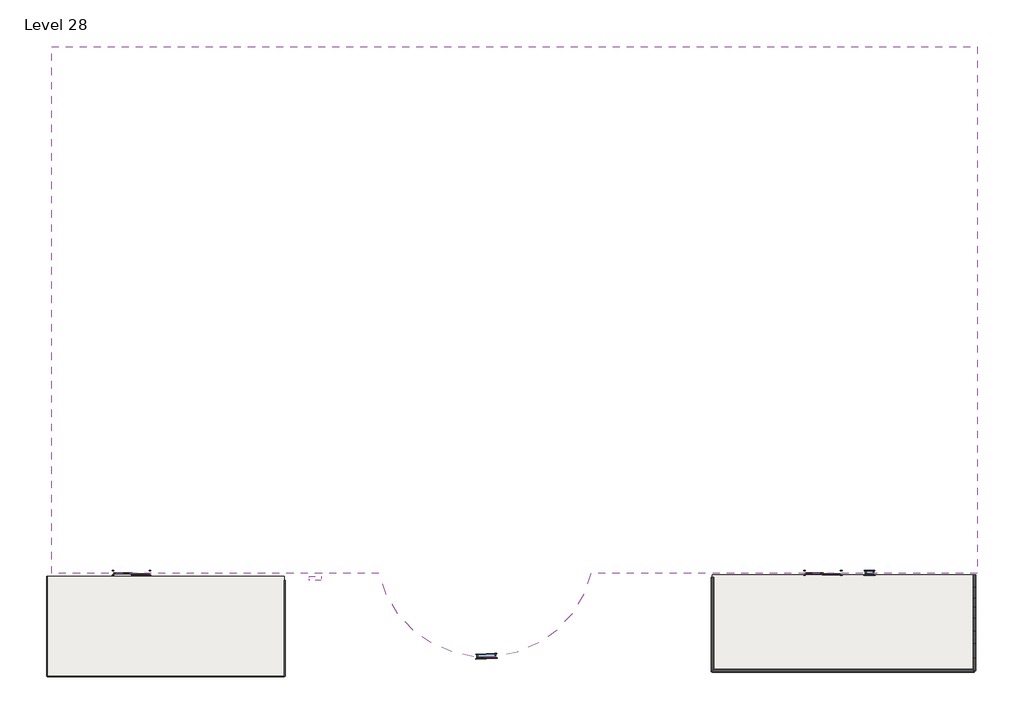
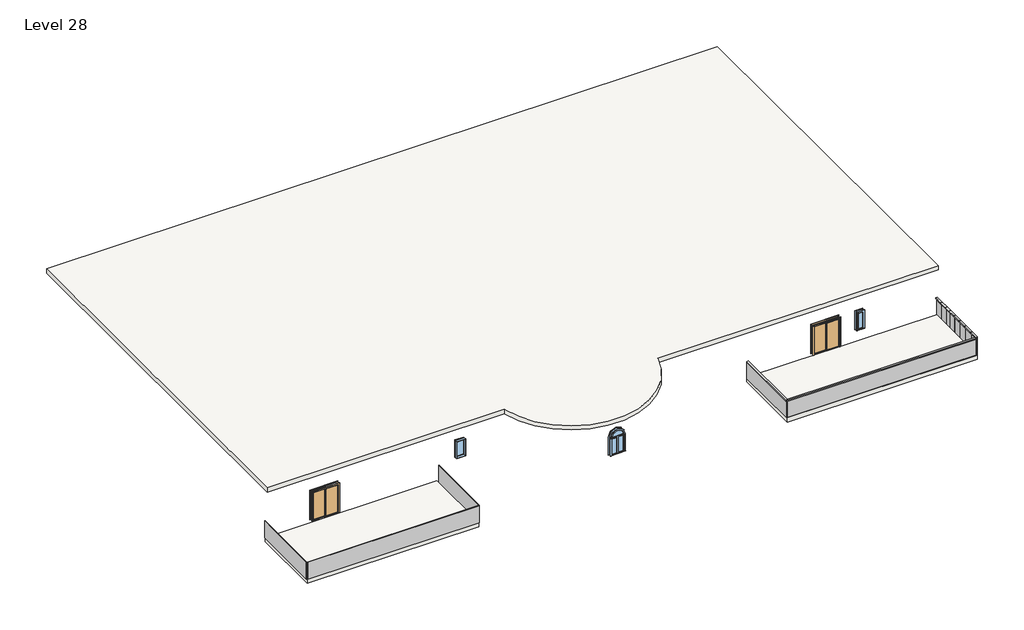
# One storey: 13 plates, 11 members, 3 slabs, 3 windows, 2 doors.
"""IFC4 building model written with IfcOpenShell, lengths in millimetres."""

from ifc_helpers import new_model, si_unit, point, frame, frame_2d, origin, place, context, project, spatial, polyline, circle_curve, trimmed, segment, composite_curve, outline, extrude, transform, mapped, element, save
from components import door_076b30e0, member_75074519, member_47bfaf8a, member_baaa0d74, member_cd3c8de8, member_7cfea1b5, member_50cacee6, member_5e365d0c, member_ae70dd35, member_19d8ec5e, system_panel_glazed_febc6b86, system_panel_glazed_7af1c9c3, system_panel_glazed_05863204, system_panel_glazed_4d5e8b0b, system_panel_glazed_a854efd3, system_panel_glazed_6a65e850, system_panel_glazed_b34e3459, system_panel_glazed_f1530dac, system_panel_glazed_53c2349a, system_panel_glazed_0853085d, system_panel_glazed_62bdce80, window_cf4adaea, window_a765b88f, window_80bd9af0

model = new_model("IFC4")

# Units and contexts
model_context = context("Model", 3, world=origin())
ifc_project = project(units=[si_unit("LENGTHUNIT", "METRE", prefix="MILLI")], contexts=[model_context])

# Site, building, storey
site = spatial("IfcSite", under=ifc_project)
building = spatial("IfcBuilding", under=site)
storey = spatial("IfcBuildingStorey", under=building, Name="Level 28", Elevation=46634.4)

# Doors
placement = place(None, origin())
door_shape = door_076b30e0(model_context)
element("IfcDoor", 1, ObjectType="Door-Double-Sliding : 68\" x 80\"", at=placement, inside=storey, context=model_context, shape_type="MappedRepresentation", body=[
    mapped(door_shape, transform((-15759.785279, -12227.7237084, 46634.4), x_axis=(-1.0, 0.0, 0.0), y_axis=(0.0, -1.0, 0.0), z_axis=(0.0, 0.0, 1.0))),
])
element("IfcDoor", 2, ObjectType="Door-Double-Sliding : 68\" x 80\"", at=placement, inside=storey, context=model_context, shape_type="MappedRepresentation", body=[
    mapped(door_shape, transform((18073.014721, -12227.7237084, 46634.4), x_axis=(-1.0, 0.0, 0.0), y_axis=(0.0, -1.0, 0.0), z_axis=(0.0, 0.0, 1.0))),
])

# Members
member_shape = member_75074519(model_context)
element("IfcMember", 3, ObjectType="Rectangular Mullion : 2.5\" x 5\" rectangular", at=placement, inside=storey, context=model_context, shape_type="MappedRepresentation", body=[
    mapped(member_shape, transform((25489.814721, -17135.5727399, 47853.6), x_axis=(1.0, 0.0, 0.0), y_axis=(0.0, 1.0, 0.0), z_axis=(0.0, 0.0, 1.0))),
])
member_2_shape = member_47bfaf8a(model_context)
element("IfcMember", 4, ObjectType="Rectangular Mullion : 2.5\" x 5\" rectangular", at=placement, inside=storey, context=model_context, shape_type="MappedRepresentation", body=[
    mapped(member_2_shape, transform((25489.814721, -15179.7727399, 47853.6), x_axis=(0.0, 0.0, 1.0), y_axis=(-1.0, 0.0, 0.0), z_axis=(0.0, -1.0, 0.0))),
])
member_3_shape = member_baaa0d74(model_context)
element("IfcMember", 5, ObjectType="Rectangular Mullion : 2.5\" x 5\" rectangular", at=placement, inside=storey, context=model_context, shape_type="MappedRepresentation", body=[
    mapped(member_3_shape, transform((12667.5594464, -12557.9237084, 47853.6), x_axis=(0.0, 0.0, 1.0), y_axis=(1.0, 0.0, 0.0), z_axis=(0.0, 1.0, 0.0))),
])
member_4_shape = member_cd3c8de8(model_context)
element("IfcMember", 6, ObjectType="Rectangular Mullion : 2.5\" x 5\" rectangular", at=placement, inside=storey, context=model_context, shape_type="MappedRepresentation", body=[
    mapped(member_4_shape, transform((25489.814721, -13030.6482241, 47853.6), x_axis=(0.0, 0.0, 1.0), y_axis=(-1.0, 0.0, 0.0), z_axis=(0.0, -1.0, 0.0))),
])
element("IfcMember", 7, ObjectType="Rectangular Mullion : 2.5\" x 5\" rectangular", at=placement, inside=storey, context=model_context, shape_type="MappedRepresentation", body=[
    mapped(member_4_shape, transform((25489.814721, -13604.9727399, 47853.6), x_axis=(0.0, 0.0, 1.0), y_axis=(-1.0, 0.0, 0.0), z_axis=(0.0, -1.0, 0.0))),
])
member_5_shape = member_7cfea1b5(model_context)
element("IfcMember", 8, ObjectType="Rectangular Mullion : 2.5\" x 5\" rectangular", at=placement, inside=storey, context=model_context, shape_type="MappedRepresentation", body=[
    mapped(member_5_shape, transform((25489.814721, -14011.3727399, 47853.6), x_axis=(0.0, 0.0, 1.0), y_axis=(-1.0, 0.0, 0.0), z_axis=(0.0, -1.0, 0.0))),
])
member_6_shape = member_50cacee6(model_context)
element("IfcMember", 9, ObjectType="Rectangular Mullion : 2.5\" x 5\" rectangular", at=placement, inside=storey, context=model_context, shape_type="MappedRepresentation", body=[
    mapped(member_6_shape, transform((25489.814721, -14570.1727399, 47853.6), x_axis=(0.0, 0.0, 1.0), y_axis=(-1.0, 0.0, 0.0), z_axis=(0.0, -1.0, 0.0))),
])
member_7_shape = member_5e365d0c(model_context)
element("IfcMember", 10, ObjectType="Rectangular Mullion : 2.5\" x 5\" rectangular", at=placement, inside=storey, context=model_context, shape_type="MappedRepresentation", body=[
    mapped(member_7_shape, transform((25489.814721, -15814.7727399, 47853.6), x_axis=(0.0, 0.0, 1.0), y_axis=(-1.0, 0.0, 0.0), z_axis=(0.0, -1.0, 0.0))),
])
member_8_shape = member_ae70dd35(model_context)
element("IfcMember", 11, ObjectType="Rectangular Mullion : 2.5\" x 5\" rectangular", at=placement, inside=storey, context=model_context, shape_type="MappedRepresentation", body=[
    mapped(member_8_shape, transform((25489.814721, -16525.9727399, 47853.6), x_axis=(0.0, 0.0, 1.0), y_axis=(-1.0, 0.0, 0.0), z_axis=(0.0, -1.0, 0.0))),
])
element("IfcMember", 12, ObjectType="Rectangular Mullion : 2.5\" x 5\" rectangular", at=placement, inside=storey, context=model_context, shape_type="MappedRepresentation", body=[
    mapped(member_2_shape, transform((25489.814721, -17135.5727399, 47853.6), x_axis=(0.0, 0.0, 1.0), y_axis=(-1.0, 0.0, 0.0), z_axis=(0.0, -1.0, 0.0))),
])
member_9_shape = member_19d8ec5e(model_context)
element("IfcMember", 13, ObjectType="Rectangular Mullion : 2.5\" x 5\" rectangular", at=placement, inside=storey, context=model_context, shape_type="MappedRepresentation", body=[
    mapped(member_9_shape, transform((12667.5594464, -17135.5727399, 47853.6), x_axis=(0.0, 0.0, 1.0), y_axis=(0.0, 1.0, 0.0), z_axis=(-1.0, 0.0, 0.0))),
])

# Plates
system_panel_glazed_shape = system_panel_glazed_febc6b86(model_context)
element("IfcPlate", 14, ObjectType="System Panel : Glazed", at=placement, inside=storey, context=model_context, shape_type="MappedRepresentation", body=[
    mapped(system_panel_glazed_shape, transform((19046.9370837, -17135.5727399, 46634.4), x_axis=(-1.0, 0.0, 0.0), y_axis=(0.0, -1.0, 0.0), z_axis=(0.0, 0.0, 1.0))),
])
system_panel_glazed_2_shape = system_panel_glazed_7af1c9c3(model_context)
element("IfcPlate", 15, ObjectType="System Panel : Glazed", at=placement, inside=storey, context=model_context, shape_type="MappedRepresentation", body=[
    mapped(system_panel_glazed_2_shape, transform((25489.814721, -16830.7727399, 46634.4), x_axis=(0.0, -1.0, 0.0), y_axis=(1.0, 0.0, 0.0), z_axis=(0.0, 0.0, 1.0))),
])
element("IfcPlate", 16, ObjectType="System Panel : Glazed", at=placement, inside=storey, context=model_context, shape_type="MappedRepresentation", body=[
    mapped(system_panel_glazed_2_shape, transform((25489.814721, -14874.9727399, 46634.4), x_axis=(0.0, -1.0, 0.0), y_axis=(1.0, 0.0, 0.0), z_axis=(0.0, 0.0, 1.0))),
])
system_panel_glazed_3_shape = system_panel_glazed_05863204(model_context)
element("IfcPlate", 17, ObjectType="System Panel : Glazed", at=placement, inside=storey, context=model_context, shape_type="MappedRepresentation", body=[
    mapped(system_panel_glazed_3_shape, transform((12667.5594464, -14846.7482241, 46634.4), x_axis=(0.0, 1.0, 0.0), y_axis=(-1.0, 0.0, 0.0), z_axis=(0.0, 0.0, 1.0))),
])
system_panel_glazed_4_shape = system_panel_glazed_4d5e8b0b(model_context)
element("IfcPlate", 18, ObjectType="System Panel : Glazed", at=placement, inside=storey, context=model_context, shape_type="MappedRepresentation", body=[
    mapped(system_panel_glazed_4_shape, transform((25489.814721, -12743.4859663, 46634.4), x_axis=(0.0, -1.0, 0.0), y_axis=(1.0, 0.0, 0.0), z_axis=(0.0, 0.0, 1.0))),
])
element("IfcPlate", 19, ObjectType="System Panel : Glazed", at=placement, inside=storey, context=model_context, shape_type="MappedRepresentation", body=[
    mapped(system_panel_glazed_4_shape, transform((25489.814721, -13317.810482, 46634.4), x_axis=(0.0, -1.0, 0.0), y_axis=(1.0, 0.0, 0.0), z_axis=(0.0, 0.0, 1.0))),
])
system_panel_glazed_5_shape = system_panel_glazed_a854efd3(model_context)
element("IfcPlate", 20, ObjectType="System Panel : Glazed", at=placement, inside=storey, context=model_context, shape_type="MappedRepresentation", body=[
    mapped(system_panel_glazed_5_shape, transform((25489.814721, -16170.3727399, 46634.4), x_axis=(0.0, -1.0, 0.0), y_axis=(1.0, 0.0, 0.0), z_axis=(0.0, 0.0, 1.0))),
])
system_panel_glazed_6_shape = system_panel_glazed_6a65e850(model_context)
element("IfcPlate", 21, ObjectType="System Panel : Glazed", at=placement, inside=storey, context=model_context, shape_type="MappedRepresentation", body=[
    mapped(system_panel_glazed_6_shape, transform((25489.814721, -15497.2727399, 46634.4), x_axis=(0.0, -1.0, 0.0), y_axis=(1.0, 0.0, 0.0), z_axis=(0.0, 0.0, 1.0))),
])
system_panel_glazed_7_shape = system_panel_glazed_b34e3459(model_context)
element("IfcPlate", 22, ObjectType="System Panel : Glazed", at=placement, inside=storey, context=model_context, shape_type="MappedRepresentation", body=[
    mapped(system_panel_glazed_7_shape, transform((25489.814721, -14290.7727399, 46634.4), x_axis=(0.0, -1.0, 0.0), y_axis=(1.0, 0.0, 0.0), z_axis=(0.0, 0.0, 1.0))),
])
system_panel_glazed_8_shape = system_panel_glazed_f1530dac(model_context)
element("IfcPlate", 23, ObjectType="System Panel : Glazed", at=placement, inside=storey, context=model_context, shape_type="MappedRepresentation", body=[
    mapped(system_panel_glazed_8_shape, transform((25489.814721, -13808.1727399, 46634.4), x_axis=(0.0, -1.0, 0.0), y_axis=(1.0, 0.0, 0.0), z_axis=(0.0, 0.0, 1.0))),
])
system_panel_glazed_9_shape = system_panel_glazed_53c2349a(model_context)
element("IfcPlate", 24, ObjectType="System Panel : Glazed", at=placement, inside=storey, context=model_context, shape_type="MappedRepresentation", body=[
    mapped(system_panel_glazed_9_shape, transform((-19874.585279, -14968.7476039, 46634.4), x_axis=(0.0, 1.0, 0.0), y_axis=(-1.0, 0.0, 0.0), z_axis=(0.0, 0.0, 1.0))),
])
system_panel_glazed_10_shape = system_panel_glazed_0853085d(model_context)
element("IfcPlate", 25, ObjectType="System Panel : Glazed", at=placement, inside=storey, context=model_context, shape_type="MappedRepresentation", body=[
    mapped(system_panel_glazed_10_shape, transform((-14083.385279, -17407.1476039, 46634.4), x_axis=(-1.0, 0.0, 0.0), y_axis=(0.0, -1.0, 0.0), z_axis=(0.0, 0.0, 1.0))),
])
system_panel_glazed_11_shape = system_panel_glazed_62bdce80(model_context)
element("IfcPlate", 26, ObjectType="System Panel : Glazed", at=placement, inside=storey, context=model_context, shape_type="MappedRepresentation", body=[
    mapped(system_panel_glazed_11_shape, transform((-8292.185279, -15062.9741674, 46634.4), x_axis=(0.0, -1.0, 0.0), y_axis=(1.0, 0.0, 0.0), z_axis=(0.0, 0.0, 1.0))),
])

# Slabs
element("IfcSlab", 27, ObjectType="Generic - 12\"", at=placement, inside=storey, context=model_context, shape_type="SweptSolid", body=[
    extrude(outline(composite_curve([segment(polyline([(25642.214721, 13428.4523961), (25642.214721, -12377.9476039), (6723.9594464, -12377.9476039)]), True, "CONTINUOUS"), segment(trimmed(circle_curve(frame_2d((1537.614721, -11147.3145626)), 5330.3498284), [point((6723.9594464, -12377.9476039))], [point((-3648.7300045, -12377.9476039))], False, "CARTESIAN"), True, "CONTINUOUS"), segment(polyline([(-3648.7300045, -12377.9476039), (-19671.385279, -12377.9476039), (-19671.385279, 13428.4523961), (25642.214721, 13428.4523961)]), True, "CONTINUOUS")], self_intersect=False)), frame((0.0, 0.0, 49719.8732819), z_axis=(0.0, 0.0, 1.0), x_axis=(1.0, 0.0, 0.0)), (0.0, 0.0, 1.0), 304.8),
])
element("IfcSlab", 28, ObjectType="Generic - 12\"", at=placement, inside=storey, context=model_context, shape_type="SweptSolid", body=[
    extrude(outline(polyline([(25489.814721, -12456.3237084), (25489.814721, -17221.8543982), (12667.5594464, -17221.8543982), (12667.5594464, -12456.3237084), (25489.814721, -12456.3237084)])), frame((0.0, 0.0, 46329.6), z_axis=(0.0, 0.0, 1.0), x_axis=(1.0, 0.0, 0.0)), (0.0, 0.0, 1.0), 304.8),
])
element("IfcSlab", 29, ObjectType="Generic - 12\"", at=placement, inside=storey, context=model_context, shape_type="SweptSolid", body=[
    extrude(outline(polyline([(-8292.185279, -12530.3476039), (-8292.185279, -17407.1476039), (-19874.585279, -17407.1476039), (-19874.585279, -12530.3476039), (-8292.185279, -12530.3476039)])), frame((0.0, 0.0, 46329.6), z_axis=(0.0, 0.0, 1.0), x_axis=(1.0, 0.0, 0.0)), (0.0, 0.0, 1.0), 304.8),
])

# Windows
window_shape = window_cf4adaea(model_context)
element("IfcWindow", 30, ObjectType="36\" x 48\"", at=placement, inside=storey, context=model_context, shape_type="MappedRepresentation", body=[
    mapped(window_shape, transform((1611.6959749, -16429.8769479, 46634.4), x_axis=(-0.9991200002820597, -0.04194311667457494, 0.0), y_axis=(0.04194311667457494, -0.9991200002820597, 0.0), z_axis=(0.0, 0.0, 1.0))),
])
window_2_shape = window_a765b88f(model_context)
element("IfcWindow", 31, ObjectType="Awning with Trim : 16\" x 48\"", at=placement, inside=storey, context=model_context, shape_type="MappedRepresentation", body=[
    mapped(window_2_shape, transform((20359.014721, -12354.7237084, 46470.5519596), x_axis=(-1.0, 0.0, 0.0), y_axis=(0.0, -1.0, 0.0), z_axis=(0.0, 0.0, 1.0))),
])
window_3_shape = window_80bd9af0(model_context)
element("IfcWindow", 32, ObjectType="Fixed : 24\" x 48\"", at=placement, inside=storey, context=model_context, shape_type="MappedRepresentation", body=[
    mapped(window_3_shape, transform((-6730.085279, -12617.2007309, 46984.5223994), x_axis=(1.0, 0.0, 0.0), y_axis=(0.0, 1.0, 0.0), z_axis=(0.0, 0.0, 1.0))),
])

save(model, "model.ifc")

# Revit data of these elements
# Type "Door-Double-Sliding : 68\" x 80\""
#   Type Mark = "10"
#   Construction Type Id = "opn-d45"
#   Assembly Code = "C1020"
#   Analytic Construction = "Wood frame, double glass door "
#   Thickness = 0' - 2"
#   Thermal Resistance (R) = 1.8150 (h·ft²·°F)/BTU
#   Heat Transfer Coefficient (U) = 0.5510 BTU/(h·ft²·°F)
#   Height = 6' - 8"
#   Rail Width = 0' - 2"
#   Stiles = 0' - 2"
#   Trim Projection Ext = 0' - 1"
#   Trim Projection Int = 0' - 1"
#   Trim Width = 0' - 3"
#   Width = 5' - 8"
#   Define Thermal Properties by = 1
#   Glazing = Glass
#   Panel Material = Wood - Birch - Solid Stained Light Low Gloss
#   Trim Material = Paint - Sienna
#   Visual Light Transmittance = 0
#   Solar Heat Gain Coefficient = 0
#   Function = (empty or 0)
#   Wall Closure = (empty or 0)
# Type "Rectangular Mullion : 2.5\" x 5\" rectangular"
#   built-in parameter 1007304 = 0.416667 (stored number, unit not read)
#   built-in parameter 1007301 = 0.104167 (stored number, unit not read)
#   built-in parameter 1007300 = 0.104167 (stored number, unit not read)
# Type "System Panel : Glazed"
#   Construction Type Id = "GSP4R"
#   Analytic Construction = "1/8 in Pilkington single glazing"
#   Visual Light Transmittance = 0.9
#   Solar Heat Gain Coefficient = 0.86
#   Heat Transfer Coefficient (U) = 1.18115 BTU/(h·ft²·°F)
# Type "Generic - 12\""
#   Assembly Code = "B1010"
#   Function = 0
#   Layers, outside or top first: 1' - 0" no material (function 1)
# Type "36\" x 48\""
#   Type Mark = "38"
#   Construction Type Id = "SGL"
#   Assembly Code = "B2020100"
#   Analytic Construction = "Large single-glazed windows"
#   Visual Light Transmittance = 0.9
#   Solar Heat Gain Coefficient = 0.86
#   Heat Transfer Coefficient (U) = 0.979472 BTU/(h·ft²·°F)
#   Height = 4' - 0"
#   Default Sill Height = 3' - 0"
#   Trim Projection - Ext. = 0' - 0 1/2"
#   Trim Projection - Int. = 0' - 0 3/4"
#   Trim Width - Exterior = 0' - 3 1/2"
#   Trim Width - Interior = 0' - 3 1/2"
#   Width = 3' - 0"
#   Window Inset = 0' - 0 3/4"
#   Define Thermal Properties by = 1
#   Glass Pane Material = Glass
#   Sash Material = Sash
#   Trim Exterior Material = Trim
#   Trim Interior Material = Trim
#   Wall Closure = (empty or 0)
# Type "Awning with Trim : 16\" x 48\""
#   Type Mark = "14"
#   Construction Type Id = "GSP4R"
#   Assembly Code = "B2020100"
#   Analytic Construction = "1/8 in Pilkington single glazing"
#   Visual Light Transmittance = 0.9
#   Solar Heat Gain Coefficient = 0.78
#   Heat Transfer Coefficient (U) = 0.6496 BTU/(h·ft²·°F)
#   Height = 4' - 0"
#   Default Sill Height = 3' - 0"
#   Trim Projection - Ext. = 0' - 0 1/2"
#   Trim Projection - Int. = 0' - 0 3/4"
#   Trim Width - Exterior = 0' - 3 1/2"
#   Trim Width - Interior = 0' - 3 1/2"
#   Width = 1' - 4"
#   Window Inset = 0' - 0 3/4"
#   Define Thermal Properties by = 1
#   Glass Pane Material = Glass
#   Sash Material = Sash
#   Trim Exterior Material = Trim
#   Trim Interior Material = Trim
#   Wall Closure = (empty or 0)
# Type "Fixed : 24\" x 48\""
#   Type Mark = "2"
#   Construction Type Id = "GSP4R"
#   Assembly Code = "B2020100"
#   Analytic Construction = "1/8 in Pilkington single glazing"
#   Visual Light Transmittance = 0.9
#   Solar Heat Gain Coefficient = 0.78
#   Heat Transfer Coefficient (U) = 0.6496 BTU/(h·ft²·°F)
#   Height = 4' - 0"
#   Default Sill Height = 3' - 0"
#   Width = 2' - 0"
#   Window Inset = 0' - 0 3/4"
#   Define Thermal Properties by = 1
#   Glass Pane Material = Glass
#   Sash Material = Sash
#   Wall Closure = (empty or 0)
# Elements 1, 2 (IfcDoor, "Door-Double-Sliding : 68\" x 80\"")
#   Phase Created = New Construction
#   Materials on its faces: "Paint - Sienna", "Wood - Birch - Solid Stained Light Low Gloss", "Glass"
# Elements 3, 4, 5, 6, 7, 8, 9, 10, 11, 12, 13 (IfcMember, "Rectangular Mullion : 2.5\" x 5\" rectangular")
#   Phase Created = New Construction
#   Materials on its faces: "Aluminum"
# Elements 14, 15, 16, 17, 18, 19, 20, 21, 22, 23, 24, 25, 26 (IfcPlate, "System Panel : Glazed")
#   Phase Created = New Construction
#   Materials on its faces: "Glass"
# Element 27 (IfcSlab, "Generic - 12\"")
#   Height Offset From Level = 11' - 1.47533"
#   Phase Created = New Construction
#   Materials on its faces: "Default Floor"
# Elements 28, 29 (IfcSlab, "Generic - 12\"")
#   Height Offset From Level = 0' - 0"
#   Phase Created = New Construction
#   Materials on its faces: "Default Floor"
# Element 30 (IfcWindow, "36\" x 48\"")
#   Mark = "20"
#   Phase Created = New Construction
#   Materials on its faces: "Sash", "Trim", "Glass"
# Element 31 (IfcWindow, "Awning with Trim : 16\" x 48\"")
#   Mark = "54"
#   Phase Created = New Construction
#   Materials on its faces: "Sash", "Trim", "Glass"
# Element 32 (IfcWindow, "Fixed : 24\" x 48\"")
#   Mark = "71"
#   Phase Created = New Construction
#   Materials on its faces: "Sash", "Glass"
# Materials
#   "Glass": class "Glass", colour RGB 0 128 192, transparency 0.75, Description = "Soda Lime Glass", Cost = 0
#   "Wood - Birch - Solid Stained Light Low Gloss": class "Wood", colour RGB 210 159 95, transparency 0, Cost = 0
#   "Paint - Sienna": colour RGB 118 70 51, transparency 0, Cost = 0
#   "Sash": class "Wood", colour RGB 224 178 126, transparency 0
#   "Trim": class "Wood", colour RGB 224 178 126, transparency 0
#   "Aluminum": class "Metal", colour RGB 247 247 247, transparency 0, Description = "Aluminum 6061", Cost = 0
#   "Default Floor": colour RGB 128 128 128, transparency 0
